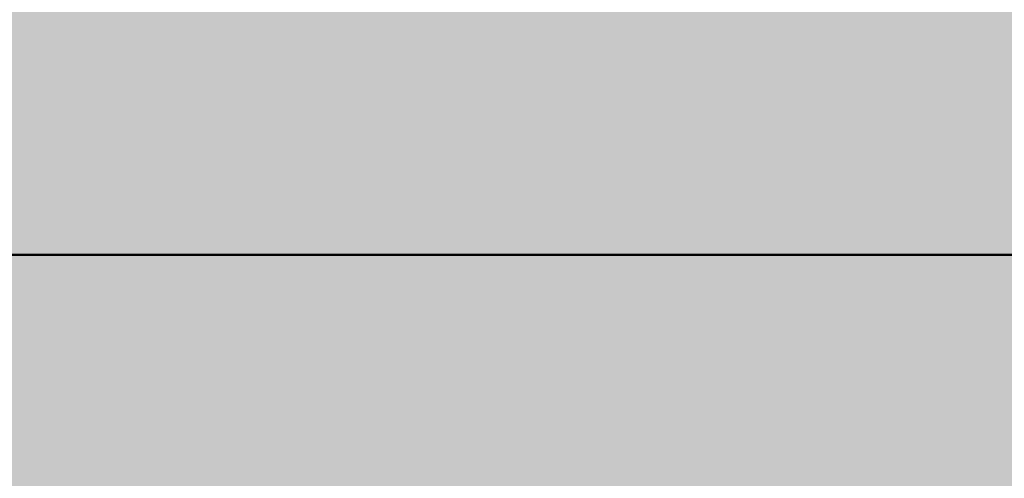
# Model space of a CAD drawing. Units: millimetres. Extents: x 0 to 2267, y 0 to 1823.
# Tile 141 of 256: x 1802 to 1823, y 1113 to 1122. Entities that reach past the tile are written whole.
import ezdxf

# ---------------------------------------------------------------- set-up
doc = ezdxf.new("R2010")
doc.units = ezdxf.units.MM
doc.header["$MEASUREMENT"] = 0
for name, color, linetype, lineweight in [('M-DIMS', 2, 'Continuous', 25), ('M-HATC', 252, 'Continuous', 18), ('M-OUTL', 7, 'Continuous', 50)]:
    doc.layers.add(name, color=color, linetype=linetype, lineweight=lineweight)
doc.styles.get("Standard").update_dxf_attribs({"font": 'arial.ttf'})
doc.dimstyles.get("Standard").update_dxf_attribs({"dimtxt": 7, "dimasz": 4, "dimexe": 0.18, "dimexo": 0.0625, "dimgap": 0.09, "dimtad": 0, "dimdec": 0, "dimzin": 0, "dimdsep": 46, "dimtxsty": 'Standard', "dimcen": 0.09, "dimadec": 0, "dimazin": 0, "dimtfac": 1, "dimtdec": 0, "dimtofl": 0, "dimtmove": 0, "dimatfit": 3, "dimfxl": 1, "dimtolj": 1, "dimtzin": 0, "dimarcsym": 0})

# ---------------------------------------------------------------- blocks, each defined once
blk = doc.blocks.new('*D1')
at = {"layer": 'Defpoints', "color": 0, "transparency": 16777216}
for p in [(1593.429, 1127.417), (1843.429, 1127.417), (1843.429, 955.628)]:
    blk.add_point(p, dxfattribs=at)
at = {"layer": 'M-DIMS', "color": 0, "lineweight": -2, "transparency": 16777216}
for p, q in [((1593.429, 1127.355), (1593.429, 955.448)), ((1843.429, 1127.355), (1843.429, 955.448)), ((1597.429, 955.628), (1710.558, 955.628)), ((1839.429, 955.628), (1726.3, 955.628))]:
    blk.add_line(p, q, dxfattribs=at)
at = {"layer": 'M-DIMS', "color": 0, "transparency": 16777216}
for points in [[(1597.429, 956.294), (1597.429, 954.961), (1593.429, 955.628)], [(1839.429, 956.294), (1839.429, 954.961), (1843.429, 955.628)]]:
    blk.add_solid(points, dxfattribs=at)
at = {"layer": 'M-DIMS', "color": 0, "transparency": 16777216, "insert": (1718.429, 955.628), "char_height": 7, "attachment_point": 5}
blk.add_mtext('\\A1;250', dxfattribs=at)

msp = doc.modelspace()

# ---------------------------------------------------------------- hatches: boundary and pattern name
at = {"layer": 'M-HATC'}
h = msp.add_hatch(color=256, dxfattribs=at)
h.dxf.hatch_style = 1
h.paths.add_polyline_path([(2065.771, 1618.062, 0.236068), (2055.771, 1638.062), (1381.087, 1638.062, 0.236068), (1371.087, 1618.062), (1371.087, 1603.062), (2055.771, 1603.062), (2065.771, 1603.062)])
h.paths.add_polyline_path([(2062.772, 1550.296), (2062.772, 1560.296), (1374.086, 1560.296), (1374.086, 1550.296), (1374.086, 1540.296), (1384.086, 1540.296), (1389.086, 1540.296), (2062.772, 1540.296)])
h.paths.add_polyline_path([(1930.929, 1282.766), (1505.929, 1282.766), (1587.628, 1235.597, 0.131652), (1600.128, 1232.247), (1836.73, 1232.247, 0.131652), (1849.23, 1235.597)])
h.paths.add_polyline_path([(1930.929, 1117.417), (1905.929, 1117.417), (1505.929, 1117.417), (1505.929, 1077.417), (1930.929, 1077.417)])
h = msp.add_hatch(color=256, dxfattribs=at)
h.dxf.hatch_style = 1
h.paths.add_polyline_path([(2055.771, 1603.062), (1381.087, 1603.062), (1381.087, 1598.062), (2055.771, 1598.062)])
h.paths.add_polyline_path([(2055.771, 1598.062), (1381.087, 1598.062), (1381.087, 1593.062), (2055.771, 1593.062)])
h.paths.add_polyline_path([(2051.307, 1536.761), (1385.55, 1536.761), (1385.55, 1526.761), (1387.55, 1526.761), (1388.537, 1525.053), (1385.332, 1521.233), (1385.332, 1521.223), (2050.254, 1522.749), (2048.321, 1525.053), (2049.307, 1526.761), (2051.307, 1526.761)])
edge = h.paths.add_edge_path()
edge.add_arc((1847.535, 1379.149), 135, 222.60306, 222.89085, ccw=False)
edge.add_line((1748.166, 1287.766), (1683.092, 1287.766))
edge.add_arc((1583.724, 1379.149), 135, 317.10915, 317.39694, ccw=False)
edge.add_arc((1678.969, 1290.671), 5, 222.8909, 317.1091, ccw=False)
edge.add_arc((1774.213, 1379.149), 135, 222.60306, 222.89085, ccw=False)
edge.add_line((1674.845, 1287.766), (1609.771, 1287.766))
edge.add_arc((1510.403, 1379.149), 135, 317.10915, 317.39694, ccw=False)
edge.add_arc((1605.647, 1290.671), 5, 222.8909, 317.1091, ccw=False)
edge.add_arc((1700.892, 1379.149), 135, 222.60306, 222.89085, ccw=False)
edge.add_line((1601.524, 1287.766), (1536.45, 1287.766))
edge.add_arc((1437.081, 1379.149), 135, 317.10915, 317.39694, ccw=False)
edge.add_arc((1532.326, 1290.671), 5, 222.8909, 317.1091, ccw=False)
edge.add_arc((1627.571, 1379.149), 135, 222.60306, 222.89085, ccw=False)
edge.add_line((1528.203, 1287.766), (1505.929, 1287.766))
edge.add_spline(control_points=[(1505.929, 1287.766), (1504.262, 1287.766), (1504.262, 1282.766), (1505.929, 1282.766)], knot_values=[0, 0, 0, 0, 5, 5, 5, 5], degree=3, periodic=0)
edge.add_line((1505.929, 1282.766), (1930.929, 1282.766))
edge.add_spline(control_points=[(1930.929, 1282.766), (1932.596, 1282.766), (1932.596, 1287.766), (1930.929, 1287.766)], knot_values=[0, 0, 0, 0, 5, 5, 5, 5], degree=3, periodic=0)
edge.add_line((1930.929, 1287.766), (1903.056, 1287.766))
edge.add_arc((1803.688, 1379.149), 135, 317.10915, 317.39694, ccw=False)
edge.add_arc((1898.932, 1290.671), 5, 222.8909, 317.1091, ccw=False)
edge.add_arc((1994.177, 1379.149), 135, 222.60306, 222.89085, ccw=False)
edge.add_line((1894.809, 1287.766), (1829.735, 1287.766))
edge.add_arc((1730.366, 1379.149), 135, 317.10915, 317.39694, ccw=False)
edge.add_arc((1825.611, 1290.671), 5, 222.8909, 317.1091, ccw=False)
edge.add_arc((1920.856, 1379.149), 135, 222.60306, 222.89085, ccw=False)
edge.add_line((1821.487, 1287.766), (1756.413, 1287.766))
edge.add_arc((1657.045, 1379.149), 135, 317.10915, 317.39694, ccw=False)
edge.add_arc((1752.29, 1290.671), 5, 222.8909, 317.1091, ccw=False)
edge = h.paths.add_edge_path()
edge.add_spline(control_points=[(1843.429, 1227.247), (1845.096, 1227.247), (1845.096, 1232.247), (1843.429, 1232.247)], knot_values=[0, 0, 0, 0, 5, 5, 5, 5], degree=3, periodic=0)
edge.add_line((1843.429, 1232.247), (1593.429, 1232.247))
edge.add_spline(control_points=[(1593.429, 1232.247), (1591.762, 1232.247), (1591.762, 1227.247), (1593.429, 1227.247)], knot_values=[0, 0, 0, 0, 5, 5, 5, 5], degree=3, periodic=0)
edge.add_line((1593.429, 1227.247), (1843.429, 1227.247))
h.paths.add_polyline_path([(1905.929, 1127.417), (1530.929, 1127.417, 0.414214), (1520.929, 1117.417), (1530.929, 1117.417), (1915.929, 1117.417, 0.414214)])
edge = h.paths.add_edge_path()
edge.add_arc((1397.086, 1498.408), 12.73, 90.7821, 190.8787, ccw=False)
edge.add_line((1396.912, 1511.136), (1428.01, 1511.349))
edge.add_line((1428.01, 1511.349), (1433.01, 1511.349))
edge.add_line((1433.01, 1511.349), (1434.439, 1511.349))
edge.add_arc((1419.474, 1498.08), 20, 41.561, 74.0821)
edge.add_line((1424.959, 1517.314), (1399.935, 1517.256))
edge.add_spline(control_points=[(1399.931, 1517.256), (1399.884, 1517.213), (1399.833, 1517.169), (1399.777, 1517.124)], knot_values=[11.567499, 11.567499, 11.567499, 11.567499, 11.814249, 11.814249, 11.814249, 11.814249], degree=3, periodic=0)
edge.add_spline(control_points=[(1399.633, 1517.01), (1399.583, 1516.972), (1399.531, 1516.934), (1399.476, 1516.895)], knot_values=[11.167718, 11.167718, 11.167718, 11.167718, 11.365188, 11.365188, 11.365188, 11.365188], degree=3, periodic=0)
edge.add_spline(control_points=[(1399.34, 1516.8), (1399.151, 1516.672), (1398.938, 1516.538), (1398.704, 1516.399)], knot_values=[10.376405, 10.376405, 10.376405, 10.376405, 11.00994, 11.00994, 11.00994, 11.00994], degree=3, periodic=0)
edge.add_spline(control_points=[(1398.657, 1516.372), (1398.579, 1516.326), (1398.498, 1516.28), (1398.415, 1516.233)], knot_values=[10.125175, 10.125175, 10.125175, 10.125175, 10.334406, 10.334406, 10.334406, 10.334406], degree=3, periodic=0)
edge.add_spline(control_points=[(1398.264, 1516.149), (1398.196, 1516.111), (1398.126, 1516.073), (1398.055, 1516.035)], knot_values=[9.832246, 9.832246, 9.832246, 9.832246, 9.999658, 9.999658, 9.999658, 9.999658], degree=3, periodic=0)
edge.add_spline(control_points=[(1397.999, 1516.005), (1397.731, 1515.862), (1397.446, 1515.717), (1397.147, 1515.571)], knot_values=[9.161808, 9.161808, 9.161808, 9.161808, 9.787769, 9.787769, 9.787769, 9.787769], degree=3, periodic=0)
edge.add_spline(control_points=[(1397.147, 1515.571), (1396.842, 1515.423), (1396.522, 1515.274), (1396.191, 1515.126)], knot_values=[8.524455, 8.524455, 8.524455, 8.524455, 9.161808, 9.161808, 9.161808, 9.161808], degree=3, periodic=0)
edge.add_spline(control_points=[(1396.078, 1515.076), (1395.985, 1515.035), (1395.892, 1514.994), (1395.798, 1514.953)], knot_values=[8.275193, 8.275193, 8.275193, 8.275193, 8.451726, 8.451726, 8.451726, 8.451726], degree=3, periodic=0)
edge.add_spline(control_points=[(1395.602, 1514.869), (1395.5, 1514.826), (1395.397, 1514.782), (1395.293, 1514.739)], knot_values=[7.962917, 7.962917, 7.962917, 7.962917, 8.152764, 8.152764, 8.152764, 8.152764], degree=3, periodic=0)
edge.add_spline(control_points=[(1395.212, 1514.706), (1394.828, 1514.547), (1394.435, 1514.393), (1394.036, 1514.244)], knot_values=[7.21254, 7.21254, 7.21254, 7.21254, 7.913148, 7.913148, 7.913148, 7.913148], degree=3, periodic=0)
edge.add_spline(control_points=[(1394.036, 1514.244), (1393.708, 1514.121), (1393.375, 1514.003), (1393.043, 1513.889)], knot_values=[6.633733, 6.633733, 6.633733, 6.633733, 7.21254, 7.21254, 7.21254, 7.21254], degree=3, periodic=0)
edge.add_spline(control_points=[(1392.821, 1513.815), (1392.72, 1513.781), (1392.618, 1513.748), (1392.517, 1513.715)], knot_values=[6.328796, 6.328796, 6.328796, 6.328796, 6.505493, 6.505493, 6.505493, 6.505493], degree=3, periodic=0)
edge.add_spline(control_points=[(1392.517, 1513.715), (1392.319, 1513.652), (1392.121, 1513.59), (1391.924, 1513.531)], knot_values=[5.984605, 5.984605, 5.984605, 5.984605, 6.328796, 6.328796, 6.328796, 6.328796], degree=3, periodic=0)
edge.add_spline(control_points=[(1391.792, 1513.491), (1391.312, 1513.35), (1390.838, 1513.224), (1390.378, 1513.117)], knot_values=[5.066697, 5.066697, 5.066697, 5.066697, 5.907055, 5.907055, 5.907055, 5.907055], degree=3, periodic=0)
edge.add_spline(control_points=[(1390.378, 1513.117), (1390.18, 1513.071), (1389.984, 1513.028), (1389.791, 1512.99)], knot_values=[4.70367, 4.70367, 4.70367, 4.70367, 5.066695, 5.066695, 5.066695, 5.066695], degree=3, periodic=0)
edge.add_spline(control_points=[(1389.422, 1512.92), (1389.246, 1512.889), (1389.073, 1512.862), (1388.904, 1512.838)], knot_values=[4.130571, 4.130571, 4.130571, 4.130571, 4.469816, 4.469816, 4.469816, 4.469816], degree=3, periodic=0)
edge.add_spline(control_points=[(1388.904, 1512.838), (1388.591, 1512.795), (1388.291, 1512.764), (1388.007, 1512.749)], knot_values=[3.504031, 3.504031, 3.504031, 3.504031, 4.130571, 4.130571, 4.130571, 4.130571], degree=3, periodic=0)
edge.add_spline(control_points=[(1387.936, 1512.746), (1387.854, 1512.742), (1387.773, 1512.74), (1387.694, 1512.739)], knot_values=[3.268866, 3.268866, 3.268866, 3.268866, 3.451164, 3.451164, 3.451164, 3.451164], degree=3, periodic=0)
edge.add_spline(control_points=[(1387.335, 1512.744), (1387.208, 1512.75), (1387.085, 1512.76), (1386.967, 1512.774)], knot_values=[2.670686, 2.670686, 2.670686, 2.670686, 2.984, 2.984, 2.984, 2.984], degree=3, periodic=0)
edge.add_spline(control_points=[(1386.833, 1512.792), (1386.821, 1512.794), (1386.809, 1512.796), (1386.797, 1512.798)], knot_values=[2.516981, 2.516981, 2.516981, 2.516981, 2.549528, 2.549528, 2.549528, 2.549528], degree=3, periodic=0)
edge.add_spline(control_points=[(1386.453, 1512.873), (1386.426, 1512.881), (1386.399, 1512.889), (1386.373, 1512.897)], knot_values=[2.095869, 2.095869, 2.095869, 2.095869, 2.17941, 2.17941, 2.17941, 2.17941], degree=3, periodic=0)
edge.add_spline(control_points=[(1386.069, 1513.019), (1386.063, 1513.022), (1386.058, 1513.025), (1386.052, 1513.028)], knot_values=[1.72453, 1.72453, 1.72453, 1.72453, 1.745933, 1.745933, 1.745933, 1.745933], degree=3, periodic=0)
edge.add_arc((1399.474, 1498.08), 20, 131.8243, 180)
edge.add_arc((1630.334, 1505.548), 250.971, 181.70518, 236.42798)
edge.add_arc((1605.34, 1483.304), 218.782, 238.66083, 243.34961)
edge.add_arc((1647.091, 1510.359), 262.899, 183.12984, 237.85344, ccw=False)
h.paths.add_polyline_path([(1406.537, 1391.964, 0.149382), (1491.551, 1296.442, -0.129517)], flags=17)
edge = h.paths.add_edge_path()
edge.add_arc((2037.384, 1498.08), 20, 0, 48.2659)
edge.add_spline(control_points=[(2050.697, 1513.005), (2050.651, 1512.985), (2050.603, 1512.966), (2050.554, 1512.948)], knot_values=[1.835652, 1.835652, 1.835652, 1.835652, 2.000781, 2.000781, 2.000781, 2.000781], degree=3, periodic=0)
edge.add_spline(control_points=[(2050.462, 1512.917), (2050.479, 1512.922), (2050.496, 1512.928), (2050.513, 1512.934)], knot_values=[2.045477, 2.045477, 2.045477, 2.045477, 2.101389, 2.101389, 2.101389, 2.101389], degree=3, periodic=0)
edge.add_spline(control_points=[(2050.129, 1512.834), (2050.198, 1512.847), (2050.266, 1512.862), (2050.331, 1512.879)], knot_values=[2.237629, 2.237629, 2.237629, 2.237629, 2.435841, 2.435841, 2.435841, 2.435841], degree=3, periodic=0)
edge.add_spline(control_points=[(2050.095, 1512.828), (2050.106, 1512.83), (2050.118, 1512.832), (2050.129, 1512.834)], knot_values=[2.435841, 2.435841, 2.435841, 2.435841, 2.468321, 2.468321, 2.468321, 2.468321], degree=3, periodic=0)
edge.add_spline(control_points=[(2049.784, 1512.785), (2049.855, 1512.792), (2049.924, 1512.801), (2049.992, 1512.811)], knot_values=[2.563852, 2.563852, 2.563852, 2.563852, 2.748541, 2.748541, 2.748541, 2.748541], degree=3, periodic=0)
edge.add_spline(control_points=[(2049.405, 1512.762), (2049.536, 1512.765), (2049.663, 1512.773), (2049.784, 1512.785)], knot_values=[2.748541, 2.748541, 2.748541, 2.748541, 3.064882, 3.064882, 3.064882, 3.064882], degree=3, periodic=0)
edge.add_spline(control_points=[(2049.17, 1512.76), (2049.234, 1512.759), (2049.297, 1512.759), (2049.358, 1512.761)], knot_values=[3.102309, 3.102309, 3.102309, 3.102309, 3.2503, 3.2503, 3.2503, 3.2503], degree=3, periodic=0)
edge.add_spline(control_points=[(2048.857, 1512.769), (2048.964, 1512.764), (2049.068, 1512.761), (2049.17, 1512.76)], knot_values=[3.2503, 3.2503, 3.2503, 3.2503, 3.486069, 3.486069, 3.486069, 3.486069], degree=3, periodic=0)
edge.add_spline(control_points=[(2048.692, 1512.779), (2048.373, 1512.801), (2048.035, 1512.841), (2047.682, 1512.897)], knot_values=[3.606429, 3.606429, 3.606429, 3.606429, 4.2989, 4.2989, 4.2989, 4.2989], degree=3, periodic=0)
edge.add_spline(control_points=[(2047.682, 1512.897), (2047.546, 1512.919), (2047.408, 1512.942), (2047.268, 1512.969)], knot_values=[4.2989, 4.2989, 4.2989, 4.2989, 4.565769, 4.565769, 4.565769, 4.565769], degree=3, periodic=0)
edge.add_spline(control_points=[(2047.268, 1512.969), (2047.145, 1512.991), (2047.021, 1513.016), (2046.895, 1513.042)], knot_values=[4.565769, 4.565769, 4.565769, 4.565769, 4.799971, 4.799971, 4.799971, 4.799971], degree=3, periodic=0)
edge.add_spline(control_points=[(2046.895, 1513.042), (2046.529, 1513.119), (2046.151, 1513.209), (2045.768, 1513.311)], knot_values=[4.799971, 4.799971, 4.799971, 4.799971, 5.483718, 5.483718, 5.483718, 5.483718], degree=3, periodic=0)
edge.add_spline(control_points=[(2045.768, 1513.311), (2045.372, 1513.415), (2044.97, 1513.532), (2044.566, 1513.659)], knot_values=[5.483718, 5.483718, 5.483718, 5.483718, 6.187866, 6.187866, 6.187866, 6.187866], degree=3, periodic=0)
edge.add_spline(control_points=[(2044.566, 1513.659), (2044.415, 1513.706), (2044.263, 1513.755), (2044.112, 1513.805)], knot_values=[6.187866, 6.187866, 6.187866, 6.187866, 6.451551, 6.451551, 6.451551, 6.451551], degree=3, periodic=0)
edge.add_spline(control_points=[(2044.112, 1513.805), (2043.997, 1513.843), (2043.882, 1513.881), (2043.767, 1513.92)], knot_values=[6.451551, 6.451551, 6.451551, 6.451551, 6.651434, 6.651434, 6.651434, 6.651434], degree=3, periodic=0)
edge.add_spline(control_points=[(2043.767, 1513.92), (2043.372, 1514.055), (2042.977, 1514.198), (2042.589, 1514.346)], knot_values=[6.651434, 6.651434, 6.651434, 6.651434, 7.338879, 7.338879, 7.338879, 7.338879], degree=3, periodic=0)
edge.add_spline(control_points=[(2042.589, 1514.346), (2042.164, 1514.507), (2041.746, 1514.675), (2041.341, 1514.846)], knot_values=[7.338879, 7.338879, 7.338879, 7.338879, 8.089209, 8.089209, 8.089209, 8.089209], degree=3, periodic=0)
edge.add_spline(control_points=[(2041.341, 1514.846), (2041.103, 1514.946), (2040.869, 1515.048), (2040.64, 1515.15)], knot_values=[8.089209, 8.089209, 8.089209, 8.089209, 8.529587, 8.529587, 8.529587, 8.529587], degree=3, periodic=0)
edge.add_spline(control_points=[(2040.51, 1515.209), (2040.082, 1515.402), (2039.675, 1515.597), (2039.295, 1515.789)], knot_values=[8.613818, 8.613818, 8.613818, 8.613818, 9.44571, 9.44571, 9.44571, 9.44571], degree=3, periodic=0)
edge.add_spline(control_points=[(2039.295, 1515.789), (2039.062, 1515.907), (2038.839, 1516.025), (2038.629, 1516.14)], knot_values=[9.44571, 9.44571, 9.44571, 9.44571, 9.956404, 9.956404, 9.956404, 9.956404], degree=3, periodic=0)
edge.add_spline(control_points=[(2038.629, 1516.14), (2038.519, 1516.2), (2038.412, 1516.26), (2038.309, 1516.319)], knot_values=[9.956404, 9.956404, 9.956404, 9.956404, 10.223542, 10.223542, 10.223542, 10.223542], degree=3, periodic=0)
edge.add_spline(control_points=[(2038.309, 1516.319), (2038.214, 1516.374), (2038.122, 1516.428), (2038.033, 1516.481)], knot_values=[10.223542, 10.223542, 10.223542, 10.223542, 10.47051, 10.47051, 10.47051, 10.47051], degree=3, periodic=0)
edge.add_spline(control_points=[(2038.033, 1516.481), (2037.786, 1516.63), (2037.564, 1516.773), (2037.372, 1516.909)], knot_values=[10.47051, 10.47051, 10.47051, 10.47051, 11.15767, 11.15767, 11.15767, 11.15767], degree=3, periodic=0)
edge.add_spline(control_points=[(2037.372, 1516.909), (2037.279, 1516.975), (2037.193, 1517.04), (2037.114, 1517.102)], knot_values=[11.15767, 11.15767, 11.15767, 11.15767, 11.49227, 11.49227, 11.49227, 11.49227], degree=3, periodic=0)
edge.add_spline(control_points=[(2036.856, 1517.326), (2036.915, 1517.269), (2036.981, 1517.21), (2037.056, 1517.149)], knot_values=[11.577341, 11.577341, 11.577341, 11.577341, 11.91035, 11.91035, 11.91035, 11.91035], degree=3, periodic=0)
edge.add_spline(control_points=[(2036.807, 1517.375), (2036.823, 1517.359), (2036.839, 1517.342), (2036.856, 1517.326)], knot_values=[11.91035, 11.91035, 11.91035, 11.91035, 12.007402, 12.007402, 12.007402, 12.007402], degree=3, periodic=0)
edge.add_spline(control_points=[(2036.702, 1517.494), (2036.71, 1517.483), (2036.72, 1517.472), (2036.729, 1517.461)], knot_values=[12.184155, 12.184155, 12.184155, 12.184155, 12.255409, 12.255409, 12.255409, 12.255409], degree=3, periodic=0)
edge.add_spline(control_points=[(2036.616, 1517.621), (2036.62, 1517.613), (2036.624, 1517.606), (2036.629, 1517.598)], knot_values=[12.487913, 12.487913, 12.487913, 12.487913, 12.541035, 12.541035, 12.541035, 12.541035], degree=3, periodic=0)
edge.add_spline(control_points=[(2036.563, 1517.786), (2036.564, 1517.779), (2036.564, 1517.773), (2036.565, 1517.766)], knot_values=[12.911761, 12.911761, 12.911761, 12.911761, 12.968286, 12.968286, 12.968286, 12.968286], degree=3, periodic=0)
edge.add_spline(control_points=[(2036.617, 1517.93), (2036.612, 1517.926), (2036.609, 1517.921), (2036.605, 1517.916)], knot_values=[13.382527, 13.382527, 13.382527, 13.382527, 13.433791, 13.433791, 13.433791, 13.433791], degree=3, periodic=0)
edge.add_spline(control_points=[(2036.749, 1518.017), (2036.736, 1518.012), (2036.724, 1518.006), (2036.712, 1518)], knot_values=[13.726299, 13.726299, 13.726299, 13.726299, 13.809928, 13.809928, 13.809928, 13.809928], degree=3, periodic=0)
edge.add_spline(control_points=[(2036.86, 1518.053), (2036.839, 1518.047), (2036.818, 1518.042), (2036.799, 1518.035)], knot_values=[13.910887, 13.910887, 13.910887, 13.910887, 14.02153, 14.02153, 14.02153, 14.02153], degree=3, periodic=0)
edge.add_line((2036.964, 1518.08), (2032.384, 1518.08))
edge.add_line((2032.384, 1518.08), (2027.384, 1518.08))
edge.add_line((2027.384, 1518.08), (2022.384, 1518.08))
edge.add_line((2022.384, 1518.08), (2017.384, 1518.08))
edge.add_arc((2017.384, 1498.08), 20, 90, 138.439)
edge.add_line((2002.419, 1511.349), (2003.848, 1511.349))
edge.add_line((2003.848, 1511.349), (2008.848, 1511.349))
edge.add_line((2008.848, 1511.349), (2039.772, 1511.138))
edge.add_arc((2039.772, 1498.408), 12.73, -10.8787, 90, ccw=False)
edge.add_arc((1789.767, 1510.359), 262.899, 302.14656, 356.87016, ccw=False)
edge.add_arc((1831.518, 1483.304), 218.782, 296.65039, 301.33917)
edge.add_arc((1806.524, 1505.548), 250.971, 303.57202, 358.29482)
h.paths.add_polyline_path([(2030.321, 1391.964, -0.129517), (1945.307, 1296.442, 0.149382)], flags=17)
edge = h.paths.add_edge_path()
edge.add_spline(control_points=[(2037.246, 1518.082), (2037.29, 1518.081), (2037.336, 1518.08), (2037.384, 1518.08)], knot_values=[0.000012, 0.000012, 0.000012, 0.000012, 0.144754, 0.144754, 0.144754, 0.144754], degree=3, periodic=0)
edge.add_line((2037.336, 1518.08), (2037.01, 1518.08))
edge.add_spline(control_points=[(2037.01, 1518.08), (2036.982, 1518.077), (2036.956, 1518.073), (2036.931, 1518.068)], knot_values=[14.13465, 14.13465, 14.13465, 14.13465, 14.247197, 14.247197, 14.247197, 14.247197], degree=3, periodic=0)
edge.add_spline(control_points=[(2036.931, 1518.068), (2036.928, 1518.067), (2036.924, 1518.067), (2036.921, 1518.066)], knot_values=[14.118315, 14.118315, 14.118315, 14.118315, 14.13465, 14.13465, 14.13465, 14.13465], degree=3, periodic=0)
edge.add_spline(control_points=[(2036.921, 1518.066), (2036.912, 1518.064), (2036.903, 1518.063), (2036.895, 1518.061)], knot_values=[14.078086, 14.078086, 14.078086, 14.078086, 14.118315, 14.118315, 14.118315, 14.118315], degree=3, periodic=0)
edge.add_spline(control_points=[(2036.895, 1518.061), (2036.883, 1518.058), (2036.872, 1518.056), (2036.86, 1518.053)], knot_values=[14.02153, 14.02153, 14.02153, 14.02153, 14.078086, 14.078086, 14.078086, 14.078086], degree=3, periodic=0)
edge.add_spline(control_points=[(2036.86, 1518.053), (2036.839, 1518.047), (2036.818, 1518.042), (2036.799, 1518.035)], knot_values=[13.910887, 13.910887, 13.910887, 13.910887, 14.02153, 14.02153, 14.02153, 14.02153], degree=3, periodic=0)
edge.add_spline(control_points=[(2036.799, 1518.035), (2036.798, 1518.035), (2036.797, 1518.035), (2036.797, 1518.035)], knot_values=[13.906906, 13.906906, 13.906906, 13.906906, 13.910887, 13.910887, 13.910887, 13.910887], degree=3, periodic=0)
edge.add_spline(control_points=[(2036.797, 1518.035), (2036.788, 1518.032), (2036.78, 1518.029), (2036.772, 1518.026)], knot_values=[13.857826, 13.857826, 13.857826, 13.857826, 13.906906, 13.906906, 13.906906, 13.906906], degree=3, periodic=0)
edge.add_spline(control_points=[(2036.772, 1518.026), (2036.764, 1518.023), (2036.756, 1518.02), (2036.749, 1518.017)], knot_values=[13.809928, 13.809928, 13.809928, 13.809928, 13.857826, 13.857826, 13.857826, 13.857826], degree=3, periodic=0)
edge.add_spline(control_points=[(2036.749, 1518.017), (2036.736, 1518.012), (2036.724, 1518.006), (2036.712, 1518)], knot_values=[13.726299, 13.726299, 13.726299, 13.726299, 13.809928, 13.809928, 13.809928, 13.809928], degree=3, periodic=0)
edge.add_spline(control_points=[(2036.712, 1518), (2036.712, 1518), (2036.712, 1518), (2036.711, 1518)], knot_values=[13.723993, 13.723993, 13.723993, 13.723993, 13.726299, 13.726299, 13.726299, 13.726299], degree=3, periodic=0)
edge.add_spline(control_points=[(2036.711, 1518), (2036.706, 1517.997), (2036.701, 1517.994), (2036.696, 1517.992)], knot_values=[13.686536, 13.686536, 13.686536, 13.686536, 13.723993, 13.723993, 13.723993, 13.723993], degree=3, periodic=0)
edge.add_spline(control_points=[(2036.696, 1517.992), (2036.692, 1517.989), (2036.687, 1517.987), (2036.683, 1517.984)], knot_values=[13.651251, 13.651251, 13.651251, 13.651251, 13.686536, 13.686536, 13.686536, 13.686536], degree=3, periodic=0)
edge.add_spline(control_points=[(2036.683, 1517.984), (2036.676, 1517.98), (2036.67, 1517.976), (2036.664, 1517.971)], knot_values=[13.596804, 13.596804, 13.596804, 13.596804, 13.651251, 13.651251, 13.651251, 13.651251], degree=3, periodic=0)
edge.add_spline(control_points=[(2036.664, 1517.971), (2036.664, 1517.971), (2036.663, 1517.971), (2036.663, 1517.971)], knot_values=[13.593956, 13.593956, 13.593956, 13.593956, 13.596804, 13.596804, 13.596804, 13.596804], degree=3, periodic=0)
edge.add_spline(control_points=[(2036.663, 1517.971), (2036.66, 1517.969), (2036.658, 1517.967), (2036.655, 1517.965)], knot_values=[13.570322, 13.570322, 13.570322, 13.570322, 13.593956, 13.593956, 13.593956, 13.593956], degree=3, periodic=0)
edge.add_spline(control_points=[(2036.655, 1517.965), (2036.653, 1517.963), (2036.65, 1517.961), (2036.647, 1517.959)], knot_values=[13.545477, 13.545477, 13.545477, 13.545477, 13.570322, 13.570322, 13.570322, 13.570322], degree=3, periodic=0)
edge.add_spline(control_points=[(2036.647, 1517.959), (2036.647, 1517.959), (2036.647, 1517.959), (2036.647, 1517.959)], knot_values=[13.543931, 13.543931, 13.543931, 13.543931, 13.545477, 13.545477, 13.545477, 13.545477], degree=3, periodic=0)
edge.add_spline(control_points=[(2036.647, 1517.959), (2036.641, 1517.954), (2036.636, 1517.949), (2036.631, 1517.945)], knot_values=[13.488237, 13.488237, 13.488237, 13.488237, 13.543931, 13.543931, 13.543931, 13.543931], degree=3, periodic=0)
edge.add_spline(control_points=[(2036.631, 1517.945), (2036.628, 1517.942), (2036.626, 1517.94), (2036.623, 1517.937)], knot_values=[13.460307, 13.460307, 13.460307, 13.460307, 13.488237, 13.488237, 13.488237, 13.488237], degree=3, periodic=0)
edge.add_spline(control_points=[(2036.623, 1517.937), (2036.622, 1517.936), (2036.62, 1517.934), (2036.618, 1517.932)], knot_values=[13.439712, 13.439712, 13.439712, 13.439712, 13.460307, 13.460307, 13.460307, 13.460307], degree=3, periodic=0)
edge.add_spline(control_points=[(2036.618, 1517.932), (2036.618, 1517.931), (2036.617, 1517.931), (2036.617, 1517.93)], knot_values=[13.433791, 13.433791, 13.433791, 13.433791, 13.439712, 13.439712, 13.439712, 13.439712], degree=3, periodic=0)
edge.add_spline(control_points=[(2036.617, 1517.93), (2036.612, 1517.926), (2036.609, 1517.921), (2036.605, 1517.916)], knot_values=[13.382527, 13.382527, 13.382527, 13.382527, 13.433791, 13.433791, 13.433791, 13.433791], degree=3, periodic=0)
edge.add_spline(control_points=[(2036.605, 1517.916), (2036.603, 1517.913), (2036.6, 1517.91), (2036.598, 1517.907)], knot_values=[13.350017, 13.350017, 13.350017, 13.350017, 13.382527, 13.382527, 13.382527, 13.382527], degree=3, periodic=0)
edge.add_spline(control_points=[(2036.598, 1517.907), (2036.597, 1517.906), (2036.596, 1517.904), (2036.595, 1517.903)], knot_values=[13.333922, 13.333922, 13.333922, 13.333922, 13.350017, 13.350017, 13.350017, 13.350017], degree=3, periodic=0)
edge.add_spline(control_points=[(2036.595, 1517.903), (2036.595, 1517.902), (2036.594, 1517.901), (2036.593, 1517.9)], knot_values=[13.323828, 13.323828, 13.323828, 13.323828, 13.333922, 13.333922, 13.333922, 13.333922], degree=3, periodic=0)
edge.add_spline(control_points=[(2036.593, 1517.9), (2036.59, 1517.895), (2036.588, 1517.891), (2036.585, 1517.886)], knot_values=[13.277545, 13.277545, 13.277545, 13.277545, 13.323828, 13.323828, 13.323828, 13.323828], degree=3, periodic=0)
edge.add_spline(control_points=[(2036.585, 1517.886), (2036.584, 1517.883), (2036.582, 1517.879), (2036.58, 1517.875)], knot_values=[13.240119, 13.240119, 13.240119, 13.240119, 13.277545, 13.277545, 13.277545, 13.277545], degree=3, periodic=0)
edge.add_spline(control_points=[(2036.58, 1517.875), (2036.58, 1517.874), (2036.579, 1517.873), (2036.578, 1517.872)], knot_values=[13.228211, 13.228211, 13.228211, 13.228211, 13.240119, 13.240119, 13.240119, 13.240119], degree=3, periodic=0)
edge.add_spline(control_points=[(2036.578, 1517.872), (2036.578, 1517.87), (2036.577, 1517.869), (2036.577, 1517.868)], knot_values=[13.215717, 13.215717, 13.215717, 13.215717, 13.228211, 13.228211, 13.228211, 13.228211], degree=3, periodic=0)
edge.add_spline(control_points=[(2036.577, 1517.868), (2036.575, 1517.864), (2036.574, 1517.86), (2036.573, 1517.857)], knot_values=[13.179847, 13.179847, 13.179847, 13.179847, 13.215717, 13.215717, 13.215717, 13.215717], degree=3, periodic=0)
edge.add_spline(control_points=[(2036.573, 1517.857), (2036.571, 1517.851), (2036.57, 1517.846), (2036.569, 1517.841)], knot_values=[13.132017, 13.132017, 13.132017, 13.132017, 13.179847, 13.179847, 13.179847, 13.179847], degree=3, periodic=0)
edge.add_spline(control_points=[(2036.569, 1517.841), (2036.568, 1517.84), (2036.568, 1517.839), (2036.568, 1517.838)], knot_values=[13.122482, 13.122482, 13.122482, 13.122482, 13.132017, 13.132017, 13.132017, 13.132017], degree=3, periodic=0)
edge.add_spline(control_points=[(2036.568, 1517.838), (2036.568, 1517.836), (2036.567, 1517.835), (2036.567, 1517.833)], knot_values=[13.105592, 13.105592, 13.105592, 13.105592, 13.122482, 13.122482, 13.122482, 13.122482], degree=3, periodic=0)
edge.add_spline(control_points=[(2036.567, 1517.833), (2036.566, 1517.829), (2036.566, 1517.826), (2036.565, 1517.822)], knot_values=[13.074063, 13.074063, 13.074063, 13.074063, 13.105592, 13.105592, 13.105592, 13.105592], degree=3, periodic=0)
edge.add_spline(control_points=[(2036.565, 1517.822), (2036.565, 1517.822), (2036.565, 1517.822), (2036.565, 1517.822)], knot_values=[13.074043, 13.074043, 13.074043, 13.074043, 13.074063, 13.074063, 13.074063, 13.074063], degree=3, periodic=0)
edge.add_spline(control_points=[(2036.565, 1517.822), (2036.564, 1517.816), (2036.564, 1517.811), (2036.564, 1517.805)], knot_values=[13.021884, 13.021884, 13.021884, 13.021884, 13.074043, 13.074043, 13.074043, 13.074043], degree=3, periodic=0)
edge.add_spline(control_points=[(2036.564, 1517.805), (2036.564, 1517.804), (2036.564, 1517.803), (2036.564, 1517.803)], knot_values=[13.01674, 13.01674, 13.01674, 13.01674, 13.021884, 13.021884, 13.021884, 13.021884], degree=3, periodic=0)
edge.add_spline(control_points=[(2036.564, 1517.803), (2036.563, 1517.801), (2036.563, 1517.798), (2036.563, 1517.796)], knot_values=[12.996438, 12.996438, 12.996438, 12.996438, 13.01674, 13.01674, 13.01674, 13.01674], degree=3, periodic=0)
edge.add_spline(control_points=[(2036.563, 1517.796), (2036.563, 1517.793), (2036.563, 1517.789), (2036.563, 1517.786)], knot_values=[12.968286, 12.968286, 12.968286, 12.968286, 12.996438, 12.996438, 12.996438, 12.996438], degree=3, periodic=0)
edge.add_spline(control_points=[(2036.563, 1517.786), (2036.564, 1517.779), (2036.564, 1517.773), (2036.565, 1517.766)], knot_values=[12.911761, 12.911761, 12.911761, 12.911761, 12.968286, 12.968286, 12.968286, 12.968286], degree=3, periodic=0)
edge.add_spline(control_points=[(2036.565, 1517.766), (2036.565, 1517.766), (2036.565, 1517.766), (2036.565, 1517.766)], knot_values=[12.911017, 12.911017, 12.911017, 12.911017, 12.911761, 12.911761, 12.911761, 12.911761], degree=3, periodic=0)
edge.add_spline(control_points=[(2036.565, 1517.766), (2036.565, 1517.762), (2036.566, 1517.759), (2036.566, 1517.756)], knot_values=[12.88528, 12.88528, 12.88528, 12.88528, 12.911017, 12.911017, 12.911017, 12.911017], degree=3, periodic=0)
edge.add_spline(control_points=[(2036.566, 1517.756), (2036.567, 1517.753), (2036.567, 1517.751), (2036.568, 1517.748)], knot_values=[12.862519, 12.862519, 12.862519, 12.862519, 12.88528, 12.88528, 12.88528, 12.88528], degree=3, periodic=0)
edge.add_spline(control_points=[(2036.568, 1517.748), (2036.568, 1517.747), (2036.568, 1517.747), (2036.568, 1517.746)], knot_values=[12.858885, 12.858885, 12.858885, 12.858885, 12.862519, 12.862519, 12.862519, 12.862519], degree=3, periodic=0)
edge.add_spline(control_points=[(2036.568, 1517.746), (2036.569, 1517.74), (2036.571, 1517.733), (2036.572, 1517.726)], knot_values=[12.8053, 12.8053, 12.8053, 12.8053, 12.858885, 12.858885, 12.858885, 12.858885], degree=3, periodic=0)
edge.add_spline(control_points=[(2036.572, 1517.726), (2036.573, 1517.723), (2036.574, 1517.719), (2036.576, 1517.715)], knot_values=[12.775176, 12.775176, 12.775176, 12.775176, 12.8053, 12.8053, 12.8053, 12.8053], degree=3, periodic=0)
edge.add_spline(control_points=[(2036.576, 1517.715), (2036.576, 1517.713), (2036.577, 1517.71), (2036.578, 1517.708)], knot_values=[12.756759, 12.756759, 12.756759, 12.756759, 12.775176, 12.775176, 12.775176, 12.775176], degree=3, periodic=0)
edge.add_spline(control_points=[(2036.578, 1517.708), (2036.578, 1517.707), (2036.578, 1517.706), (2036.579, 1517.705)], knot_values=[12.748742, 12.748742, 12.748742, 12.748742, 12.756759, 12.756759, 12.756759, 12.756759], degree=3, periodic=0)
edge.add_spline(control_points=[(2036.579, 1517.705), (2036.581, 1517.698), (2036.583, 1517.692), (2036.586, 1517.685)], knot_values=[12.69959, 12.69959, 12.69959, 12.69959, 12.748742, 12.748742, 12.748742, 12.748742], degree=3, periodic=0)
edge.add_spline(control_points=[(2036.586, 1517.685), (2036.588, 1517.68), (2036.59, 1517.675), (2036.592, 1517.669)], knot_values=[12.659038, 12.659038, 12.659038, 12.659038, 12.69959, 12.69959, 12.69959, 12.69959], degree=3, periodic=0)
edge.add_spline(control_points=[(2036.592, 1517.669), (2036.594, 1517.665), (2036.596, 1517.66), (2036.598, 1517.656)], knot_values=[12.626806, 12.626806, 12.626806, 12.626806, 12.659038, 12.659038, 12.659038, 12.659038], degree=3, periodic=0)
edge.add_spline(control_points=[(2036.598, 1517.656), (2036.598, 1517.655), (2036.599, 1517.654), (2036.599, 1517.653)], knot_values=[12.619394, 12.619394, 12.619394, 12.619394, 12.626806, 12.626806, 12.626806, 12.626806], degree=3, periodic=0)
edge.add_spline(control_points=[(2036.599, 1517.653), (2036.604, 1517.642), (2036.61, 1517.632), (2036.616, 1517.621)], knot_values=[12.541039, 12.541039, 12.541039, 12.541039, 12.619394, 12.619394, 12.619394, 12.619394], degree=3, periodic=0)
edge.add_spline(control_points=[(2036.616, 1517.621), (2036.616, 1517.621), (2036.616, 1517.621), (2036.616, 1517.621)], knot_values=[12.541035, 12.541035, 12.541035, 12.541035, 12.541039, 12.541039, 12.541039, 12.541039], degree=3, periodic=0)
edge.add_spline(control_points=[(2036.616, 1517.621), (2036.62, 1517.613), (2036.624, 1517.606), (2036.629, 1517.598)], knot_values=[12.487913, 12.487913, 12.487913, 12.487913, 12.541035, 12.541035, 12.541035, 12.541035], degree=3, periodic=0)
edge.add_spline(control_points=[(2036.629, 1517.598), (2036.633, 1517.592), (2036.637, 1517.585), (2036.641, 1517.579)], knot_values=[12.443982, 12.443982, 12.443982, 12.443982, 12.487913, 12.487913, 12.487913, 12.487913], degree=3, periodic=0)
edge.add_spline(control_points=[(2036.641, 1517.579), (2036.641, 1517.578), (2036.642, 1517.576), (2036.643, 1517.575)], knot_values=[12.434996, 12.434996, 12.434996, 12.434996, 12.443982, 12.443982, 12.443982, 12.443982], degree=3, periodic=0)
edge.add_spline(control_points=[(2036.643, 1517.575), (2036.653, 1517.56), (2036.664, 1517.544), (2036.676, 1517.528)], knot_values=[12.329647, 12.329647, 12.329647, 12.329647, 12.434996, 12.434996, 12.434996, 12.434996], degree=3, periodic=0)
edge.add_spline(control_points=[(2036.676, 1517.528), (2036.684, 1517.517), (2036.693, 1517.505), (2036.702, 1517.494)], knot_values=[12.255409, 12.255409, 12.255409, 12.255409, 12.329647, 12.329647, 12.329647, 12.329647], degree=3, periodic=0)
edge.add_spline(control_points=[(2036.702, 1517.494), (2036.71, 1517.483), (2036.72, 1517.472), (2036.729, 1517.461)], knot_values=[12.184155, 12.184155, 12.184155, 12.184155, 12.255409, 12.255409, 12.255409, 12.255409], degree=3, periodic=0)
edge.add_spline(control_points=[(2036.729, 1517.461), (2036.744, 1517.444), (2036.759, 1517.426), (2036.775, 1517.409)], knot_values=[12.075961, 12.075961, 12.075961, 12.075961, 12.184155, 12.184155, 12.184155, 12.184155], degree=3, periodic=0)
edge.add_spline(control_points=[(2036.775, 1517.409), (2036.776, 1517.407), (2036.777, 1517.406), (2036.778, 1517.405)], knot_values=[12.069502, 12.069502, 12.069502, 12.069502, 12.075961, 12.075961, 12.075961, 12.075961], degree=3, periodic=0)
edge.add_spline(control_points=[(2036.778, 1517.405), (2036.788, 1517.395), (2036.797, 1517.385), (2036.807, 1517.375)], knot_values=[12.007402, 12.007402, 12.007402, 12.007402, 12.069502, 12.069502, 12.069502, 12.069502], degree=3, periodic=0)
edge.add_spline(control_points=[(2036.807, 1517.375), (2036.823, 1517.359), (2036.839, 1517.342), (2036.856, 1517.326)], knot_values=[11.91035, 11.91035, 11.91035, 11.91035, 12.007402, 12.007402, 12.007402, 12.007402], degree=3, periodic=0)
edge.add_spline(control_points=[(2036.856, 1517.326), (2036.915, 1517.269), (2036.981, 1517.21), (2037.056, 1517.149)], knot_values=[11.577341, 11.577341, 11.577341, 11.577341, 11.91035, 11.91035, 11.91035, 11.91035], degree=3, periodic=0)
edge.add_spline(control_points=[(2037.056, 1517.149), (2037.075, 1517.134), (2037.094, 1517.118), (2037.114, 1517.102)], knot_values=[11.49227, 11.49227, 11.49227, 11.49227, 11.577341, 11.577341, 11.577341, 11.577341], degree=3, periodic=0)
edge.add_spline(control_points=[(2037.114, 1517.102), (2037.193, 1517.04), (2037.279, 1516.975), (2037.372, 1516.909)], knot_values=[11.15767, 11.15767, 11.15767, 11.15767, 11.49227, 11.49227, 11.49227, 11.49227], degree=3, periodic=0)
edge.add_spline(control_points=[(2037.372, 1516.909), (2037.564, 1516.773), (2037.786, 1516.63), (2038.033, 1516.481)], knot_values=[10.47051, 10.47051, 10.47051, 10.47051, 11.15767, 11.15767, 11.15767, 11.15767], degree=3, periodic=0)
edge.add_spline(control_points=[(2038.033, 1516.481), (2038.122, 1516.428), (2038.214, 1516.374), (2038.309, 1516.319)], knot_values=[10.223542, 10.223542, 10.223542, 10.223542, 10.47051, 10.47051, 10.47051, 10.47051], degree=3, periodic=0)
edge.add_spline(control_points=[(2038.309, 1516.319), (2038.412, 1516.26), (2038.519, 1516.2), (2038.629, 1516.14)], knot_values=[9.956404, 9.956404, 9.956404, 9.956404, 10.223542, 10.223542, 10.223542, 10.223542], degree=3, periodic=0)
edge.add_spline(control_points=[(2038.629, 1516.14), (2038.839, 1516.025), (2039.062, 1515.907), (2039.295, 1515.789)], knot_values=[9.44571, 9.44571, 9.44571, 9.44571, 9.956404, 9.956404, 9.956404, 9.956404], degree=3, periodic=0)
edge.add_spline(control_points=[(2039.295, 1515.789), (2039.675, 1515.597), (2040.082, 1515.402), (2040.51, 1515.209)], knot_values=[8.613818, 8.613818, 8.613818, 8.613818, 9.44571, 9.44571, 9.44571, 9.44571], degree=3, periodic=0)
edge.add_spline(control_points=[(2040.51, 1515.209), (2040.553, 1515.189), (2040.597, 1515.17), (2040.64, 1515.15)], knot_values=[8.529587, 8.529587, 8.529587, 8.529587, 8.613818, 8.613818, 8.613818, 8.613818], degree=3, periodic=0)
edge.add_spline(control_points=[(2040.64, 1515.15), (2040.869, 1515.048), (2041.103, 1514.946), (2041.341, 1514.846)], knot_values=[8.089209, 8.089209, 8.089209, 8.089209, 8.529587, 8.529587, 8.529587, 8.529587], degree=3, periodic=0)
edge.add_spline(control_points=[(2041.341, 1514.846), (2041.746, 1514.675), (2042.164, 1514.507), (2042.589, 1514.346)], knot_values=[7.338879, 7.338879, 7.338879, 7.338879, 8.089209, 8.089209, 8.089209, 8.089209], degree=3, periodic=0)
edge.add_spline(control_points=[(2042.589, 1514.346), (2042.977, 1514.198), (2043.372, 1514.055), (2043.767, 1513.92)], knot_values=[6.651434, 6.651434, 6.651434, 6.651434, 7.338879, 7.338879, 7.338879, 7.338879], degree=3, periodic=0)
edge.add_spline(control_points=[(2043.767, 1513.92), (2043.882, 1513.881), (2043.997, 1513.843), (2044.112, 1513.805)], knot_values=[6.451551, 6.451551, 6.451551, 6.451551, 6.651434, 6.651434, 6.651434, 6.651434], degree=3, periodic=0)
edge.add_spline(control_points=[(2044.112, 1513.805), (2044.263, 1513.755), (2044.415, 1513.706), (2044.566, 1513.659)], knot_values=[6.187866, 6.187866, 6.187866, 6.187866, 6.451551, 6.451551, 6.451551, 6.451551], degree=3, periodic=0)
edge.add_spline(control_points=[(2044.566, 1513.659), (2044.97, 1513.532), (2045.372, 1513.415), (2045.768, 1513.311)], knot_values=[5.483718, 5.483718, 5.483718, 5.483718, 6.187866, 6.187866, 6.187866, 6.187866], degree=3, periodic=0)
edge.add_spline(control_points=[(2045.768, 1513.311), (2046.151, 1513.209), (2046.529, 1513.119), (2046.895, 1513.042)], knot_values=[4.799971, 4.799971, 4.799971, 4.799971, 5.483718, 5.483718, 5.483718, 5.483718], degree=3, periodic=0)
edge.add_spline(control_points=[(2046.895, 1513.042), (2047.021, 1513.016), (2047.145, 1512.991), (2047.268, 1512.969)], knot_values=[4.565769, 4.565769, 4.565769, 4.565769, 4.799971, 4.799971, 4.799971, 4.799971], degree=3, periodic=0)
edge.add_spline(control_points=[(2047.268, 1512.969), (2047.408, 1512.942), (2047.546, 1512.919), (2047.682, 1512.897)], knot_values=[4.2989, 4.2989, 4.2989, 4.2989, 4.565769, 4.565769, 4.565769, 4.565769], degree=3, periodic=0)
edge.add_spline(control_points=[(2047.682, 1512.897), (2048.035, 1512.841), (2048.373, 1512.801), (2048.692, 1512.779)], knot_values=[3.606429, 3.606429, 3.606429, 3.606429, 4.2989, 4.2989, 4.2989, 4.2989], degree=3, periodic=0)
edge.add_spline(control_points=[(2048.692, 1512.779), (2048.748, 1512.775), (2048.803, 1512.772), (2048.857, 1512.769)], knot_values=[3.486069, 3.486069, 3.486069, 3.486069, 3.606429, 3.606429, 3.606429, 3.606429], degree=3, periodic=0)
edge.add_spline(control_points=[(2048.857, 1512.769), (2048.964, 1512.764), (2049.068, 1512.761), (2049.17, 1512.76)], knot_values=[3.2503, 3.2503, 3.2503, 3.2503, 3.486069, 3.486069, 3.486069, 3.486069], degree=3, periodic=0)
edge.add_spline(control_points=[(2049.17, 1512.76), (2049.234, 1512.759), (2049.297, 1512.759), (2049.358, 1512.761)], knot_values=[3.102309, 3.102309, 3.102309, 3.102309, 3.2503, 3.2503, 3.2503, 3.2503], degree=3, periodic=0)
edge.add_spline(control_points=[(2049.358, 1512.761), (2049.374, 1512.761), (2049.39, 1512.761), (2049.405, 1512.762)], knot_values=[3.064882, 3.064882, 3.064882, 3.064882, 3.102309, 3.102309, 3.102309, 3.102309], degree=3, periodic=0)
edge.add_spline(control_points=[(2049.405, 1512.762), (2049.536, 1512.765), (2049.663, 1512.773), (2049.784, 1512.785)], knot_values=[2.748541, 2.748541, 2.748541, 2.748541, 3.064882, 3.064882, 3.064882, 3.064882], degree=3, periodic=0)
edge.add_spline(control_points=[(2049.784, 1512.785), (2049.855, 1512.792), (2049.924, 1512.801), (2049.992, 1512.811)], knot_values=[2.563852, 2.563852, 2.563852, 2.563852, 2.748541, 2.748541, 2.748541, 2.748541], degree=3, periodic=0)
edge.add_spline(control_points=[(2049.992, 1512.811), (2050.026, 1512.816), (2050.061, 1512.822), (2050.095, 1512.828)], knot_values=[2.468321, 2.468321, 2.468321, 2.468321, 2.563852, 2.563852, 2.563852, 2.563852], degree=3, periodic=0)
edge.add_spline(control_points=[(2050.095, 1512.828), (2050.106, 1512.83), (2050.118, 1512.832), (2050.129, 1512.834)], knot_values=[2.435841, 2.435841, 2.435841, 2.435841, 2.468321, 2.468321, 2.468321, 2.468321], degree=3, periodic=0)
edge.add_spline(control_points=[(2050.129, 1512.834), (2050.198, 1512.847), (2050.266, 1512.862), (2050.331, 1512.879)], knot_values=[2.237629, 2.237629, 2.237629, 2.237629, 2.435841, 2.435841, 2.435841, 2.435841], degree=3, periodic=0)
edge.add_spline(control_points=[(2050.331, 1512.879), (2050.375, 1512.891), (2050.419, 1512.903), (2050.462, 1512.917)], knot_values=[2.101389, 2.101389, 2.101389, 2.101389, 2.237629, 2.237629, 2.237629, 2.237629], degree=3, periodic=0)
edge.add_spline(control_points=[(2050.462, 1512.917), (2050.479, 1512.922), (2050.496, 1512.928), (2050.513, 1512.934)], knot_values=[2.045477, 2.045477, 2.045477, 2.045477, 2.101389, 2.101389, 2.101389, 2.101389], degree=3, periodic=0)
edge.add_spline(control_points=[(2050.513, 1512.934), (2050.527, 1512.938), (2050.54, 1512.943), (2050.554, 1512.948)], knot_values=[2.000781, 2.000781, 2.000781, 2.000781, 2.045477, 2.045477, 2.045477, 2.045477], degree=3, periodic=0)
edge.add_spline(control_points=[(2050.554, 1512.948), (2050.603, 1512.966), (2050.651, 1512.985), (2050.697, 1513.005)], knot_values=[1.835652, 1.835652, 1.835652, 1.835652, 2.000781, 2.000781, 2.000781, 2.000781], degree=3, periodic=0)
edge.add_arc((2037.384, 1498.08), 20, 48.2659, 90.1299)
edge = h.paths.add_edge_path(flags=16)
edge.add_spline(control_points=[(1386.139, 1512.986), (1388.92, 1511.739), (1398.039, 1515.519), (1399.931, 1517.256)], knot_values=[1.831046, 1.831046, 1.831046, 1.831046, 11.814249, 11.814249, 11.814249, 11.814249], degree=3, periodic=0)
edge.add_line((1399.931, 1517.256), (1393.743, 1517.242))
edge.add_arc((1399.474, 1498.08), 20, 106.6501, 131.8173)

# ---------------------------------------------------------------- linework, layer by layer
at = {"layer": 'M-OUTL'}
for p, q in [((1505.929, 1117.417), (1930.929, 1117.417)), ((1718.429, 1117.417), (1843.429, 1117.417))]:
    msp.add_line(p, q, dxfattribs=at)

# ---------------------------------------------------------------- dimensions: what is measured, and where the dimension line sits
at = {"layer": 'M-DIMS'}
dim = msp.add_linear_dim(base=(1843.429, 955.628), p1=(1593.429, 1127.417), p2=(1843.429, 1127.417), dimstyle='Standard', override={"dimclrd": 0, "dimclre": 0, "dimclrt": 0}, dxfattribs=at)
dim.commit()
dim.dimension.update_dxf_attribs({"geometry": '*D1', "text_midpoint": (1718.429, 955.628)})

doc.saveas('drawing.dxf')
